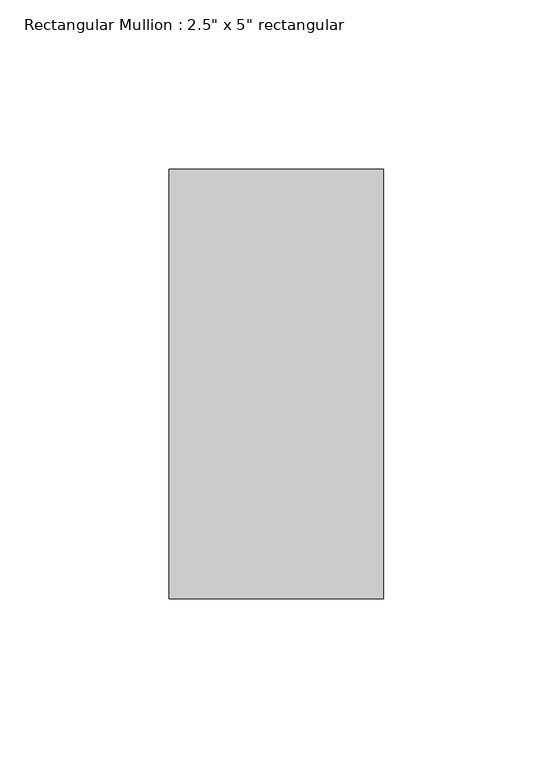
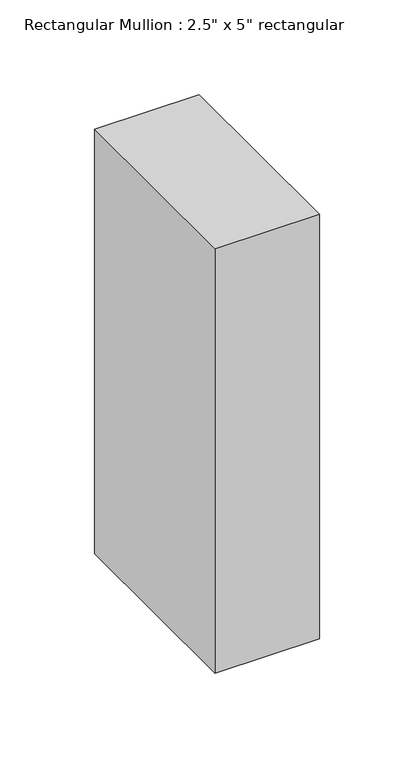
"""IFC4 building model written with IfcOpenShell, lengths in millimetres: member geometry."""

from ifc_helpers import new_model, si_unit, frame, origin, place, context, project, spatial, polyline, outline, extrude, source, transform, mapped, element, save


def member_5d67b9fc(model_context):
    return source(origin(), model_context, "Body", "SweptSolid", [
        extrude(outline(polyline([(31.75, 63.5), (31.75, -63.5), (-31.75, -63.5), (-31.75, 63.5), (31.75, 63.5)])), frame((0.0, 0.0, -273.05), z_axis=(0.0, 0.0, 1.0), x_axis=(1.0, 0.0, 0.0)), (0.0, 0.0, 1.0), 273.05),
    ])


if __name__ == "__main__":
    model = new_model("IFC4")
    model_context = context("Model", 3, world=origin())
    ifc_project = project(units=[si_unit("LENGTHUNIT", "METRE", prefix="MILLI")], contexts=[model_context])
    site = spatial("IfcSite", under=ifc_project)
    building = spatial("IfcBuilding", under=site)
    placement = place(None, origin())
    member_shape = member_5d67b9fc(model_context)
    element("IfcMember", 1, ObjectType="Rectangular Mullion : 2.5\" x 5\" rectangular", at=placement, inside=building, context=model_context, shape_type="MappedRepresentation", body=[
        mapped(member_shape, transform((0.0, 0.0, 0.0), x_axis=(1.0, 0.0, 0.0), y_axis=(0.0, 1.0, 0.0), z_axis=(0.0, 0.0, 1.0))),
    ])
    save(model, "model.ifc")

# Revit data of these elements
# Type "Rectangular Mullion : 2.5\" x 5\" rectangular"
#   built-in parameter 1007304 = 0.416667 (stored number, unit not read)
#   built-in parameter 1007301 = 0.104167 (stored number, unit not read)
#   built-in parameter 1007300 = 0.104167 (stored number, unit not read)
# Element 1 (IfcMember, "Rectangular Mullion : 2.5\" x 5\" rectangular")
#   Materials on its faces: "Aluminum"
# Materials
#   "Aluminum": class "Metal", colour RGB 247 247 247, transparency 0, Description = "Aluminum 6061", Cost = 0
